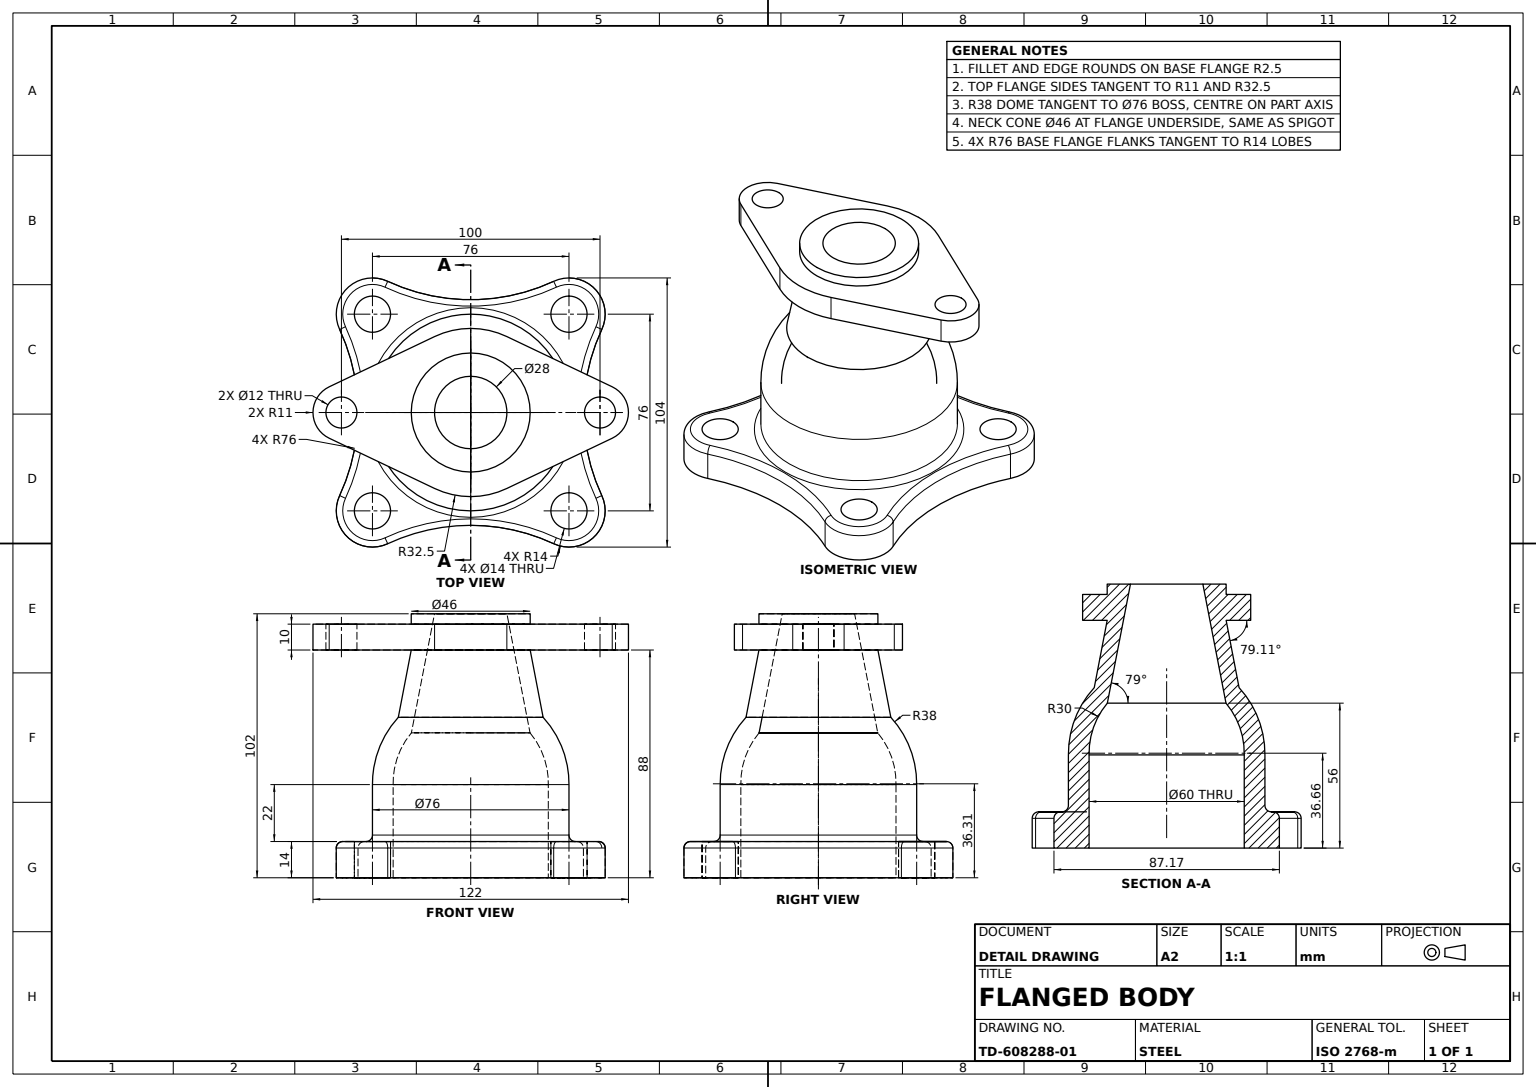
SolidWorks part; units mm, degrees
material "Plain Carbon Steel"
ref_plane "Front Plane" through (0, 0, 0) normal (0, 0, 1) x (1, 0, 0)
ref_plane "Top Plane" through (0, 0, 0) normal (0, 1, 0) x (1, 0, 0)
ref_plane "Right Plane" through (0, 0, 0) normal (1, 0, 0) x (0, 0, -1)
sketch "Base Flange Sketch" plane through (0, 0, 0) normal (0, 1, 0) x (1, 0, 0)
  line L0 (0, 0) -> (11.2434, 0) construction
  line L1 (0, 0) -> (0, 14.5705) construction
  circle A0 centre (0, 0) radius 38 construction
  arc A1 (-32.0889, 50.6909) -> (-50.6909, 32.0889) centre (-38, 38) ccw
  arc A2 (50.6909, 32.0889) -> (32.0889, 50.6909) centre (38, 38) ccw
  arc A3 (-50.6909, -32.0889) -> (-32.0889, -50.6909) centre (-38, -38) ccw
  arc A4 (32.0889, -50.6909) -> (50.6909, -32.0889) centre (38, -38) ccw
  arc A5 (-32.0889, 50.6909) -> (32.0889, 50.6909) centre (0, 119.5843) ccw
  arc A6 (-50.6909, 32.0889) -> (-50.6909, -32.0889) centre (-119.5843, 0) cw
  arc A7 (-32.0889, -50.6909) -> (32.0889, -50.6909) centre (0, -119.5843) cw
  arc A8 (50.6909, 32.0889) -> (50.6909, -32.0889) centre (119.5843, 0) ccw
  dimension "D1" = 76
  dimension "D2" = 28
  dimension "D5" = 76
  dimension "D6" = 76
  dimension "D7" = 76
  dimension "D3" = 76
  dimension "D4" = 76
extrude "Base Flange" add sketch "Base Flange Sketch" along normal blind 14
sketch "Base Boss Sketch" plane through (0, 14, 0) normal (0, 1, 0) x (1, 0, 0)
  circle A0 centre (0, 0) radius 38
  dimension "D1" = 76
extrude "Base Boss Ø76" add sketch "Base Boss Sketch" along normal blind 22
sketch "Ball Body Profile" plane through (0, 0, 0) normal (1, 0, 0) x (0, 0, -1)
  line L0 (0, 14) -> (0, 62) construction
  line L1 (32.0889, 14) -> (-32.0889, 14) construction
  line L2 (0, 62) -> (-28, 62)
  line L3 (0, 36) -> (-38, 36)
  line L4 (38, 36) -> (-38, 36) construction
  line L5 (0, 62) -> (0, 36)
  arc A0 (-38, 36) -> (-28, 62) centre (-0.0012, 36.3082) cw
  dimension "D2" = 38
  dimension "D1" = 0.0012
  dimension "D3" = 28
  dimension "D4" = 38
revolve "Ball Body" add sketch "Ball Body Profile" angle 360 about L0
sketch "Neck Loft Lower Profile" plane through (0, 62, 0) normal (0, 1, 0) x (1, 0, 0)
  circle A0 centre (0, 0) radius 28 construction
  circle A1 centre (0, 0) radius 28
ref_plane "Neck Top Plane" through (0, 88, 0) normal (0, 1, 0) x (1, 0, 0)
sketch "Neck Loft Upper Profile Ø46" plane through (0, 88, 0) normal (0, 1, 0) x (1, 0, 0)
  circle A0 centre (0, 0) radius 23
  dimension "D1" = 46
loft "Neck Loft" add profiles "Neck Loft Upper Profile Ø46", "Neck Loft Lower Profile"
sketch "Top Flange Sketch" plane through (0, 88, 0) normal (0, 1, 0) x (1, 0, 0)
  line L0 (0, 0) -> (0, -5.9991) construction
  line L1 (-54.73, 9.9311) -> (-13.975, 29.3419)
  line L2 (-54.73, -9.9311) -> (-13.975, -29.3419)
  line L3 (13.975, 29.3419) -> (54.73, 9.9311)
  line L4 (13.975, -29.3419) -> (54.73, -9.9311)
  arc A0 (-13.975, -29.3419) -> (13.975, -29.3419) centre (0, 0) ccw
  arc A1 (54.73, -9.9311) -> (54.73, 9.9311) centre (50, 0) ccw
  arc A2 (-54.73, 9.9311) -> (-54.73, -9.9311) centre (-50, 0) ccw
  arc A4 (13.975, 29.3419) -> (-13.975, 29.3419) centre (0, 0) ccw
  dimension "D1" = 65
  dimension "D2" = 22
  dimension "D3" = 100
extrude "Top Flange" add sketch "Top Flange Sketch" along normal blind 10
sketch "Top Spigot Sketch" plane through (0, 98, 0) normal (0, 1, 0) x (1, 0, 0)
  circle A0 centre (0, 0) radius 23
  dimension "D1" = 46
extrude "Top Spigot Ø46" add sketch "Top Spigot Sketch" along normal blind 4
sketch "Ball Groove Profile" plane through (0, 0, 0) normal (0, 0, 1) x (1, 0, 0)
  line L0 (0, 102) -> (0, 36) construction
  line L1 (0, 102) -> (14, 102)
  line L2 (14, 102) -> (22.9415, 56)
  line L3 (23, 102) -> (-23, 102) construction
  line L4 (38, 36) -> (-38, 36) construction
  line L5 (22.9415, 56) -> (0, 56)
  line L6 (0, 102) -> (0, 56)
  dimension "D1" = 20
  dimension "D2" = 14
  dimension "D3" = 11
revolve "Ball Groove" cut sketch "Ball Groove Profile" angle 360 about L0
sketch "Inner Cavity Profile" plane through (0, 0, 0) normal (0, 0, 1) x (1, 0, 0)
  line L0 (0, 56) -> (0, 36) construction
  line L1 (22.9415, 56) -> (-22.9415, 56) construction
  line L2 (0, 36) -> (30, 36)
  line L3 (38, 36) -> (-38, 36) construction
  line L4 (22.9415, 56) -> (0, 56)
  line L5 (0, 56) -> (0, 36)
  arc A0 (30, 36) -> (22.9415, 56) centre (0.0073, 36.6604) ccw
  dimension "D2" = 30
  dimension "D1" = 30
  dimension "D3" = 0.0073
revolve "Inner Cavity" cut sketch "Inner Cavity Profile" angle 360 about L0
sketch "Bottom Bore Sketch" plane through (0, 36, 0) normal (0, 1, 0) x (1, 0, 0)
  circle A0 centre (0, 0) radius 30
  dimension "D1" = 60
extrude "Bottom Bore Ø60" cut sketch "Bottom Bore Sketch" against normal through all
sketch "Base Mounting Holes Sketch" plane through (0, 14, 0) normal (0, 1, 0) x (1, 0, 0)
  circle A0 centre (38, 38) radius 7
  circle A1 centre (38, -38) radius 7
  circle A2 centre (-38, 38) radius 7
  circle A3 centre (-38, -38) radius 7
  dimension "D1" = 14
extrude "Base Mounting Holes 4xØ14" cut sketch "Base Mounting Holes Sketch" against normal through all
sketch "Top Flange Holes Sketch" plane through (0, 98, 0) normal (0, 1, 0) x (1, 0, 0)
  circle A0 centre (50, 0) radius 6
  circle A1 centre (-50, 0) radius 6
  dimension "D1" = 12
extrude "Top Flange Holes 2xØ12" cut sketch "Top Flange Holes Sketch" against normal up to next
fillet "Base Boss Fillet R2.5" radius 2.5 9 edges at (-47.8995, 14, -47.8995) (0, 14, -43.5843) (47.8995, 14, -47.8995) (43.5843, 14, 0) (47.8995, 14, 47.8995) (0, 14, 43.5843) (-47.8995, 14, 47.8995) (0, 14, 38) (-43.5843, 14, 0)
